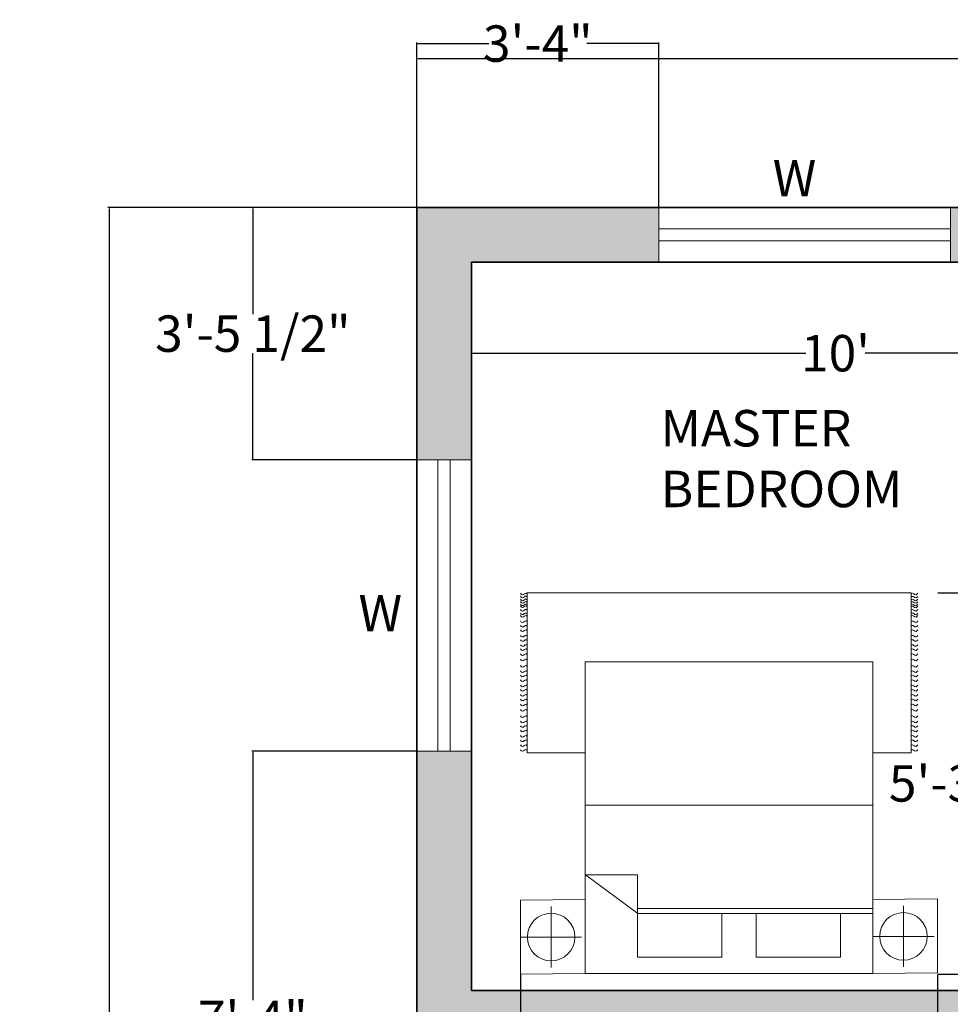
# Model space of a CAD drawing. Units: inches. Extents: x 302 to 1258, y 831 to 1373.
# Tile 9 of 13: x 781 to 934, y 1211 to 1373. Entities that reach past the tile are written whole.
import ezdxf

# ---------------------------------------------------------------- set-up
doc = ezdxf.new("R2010")
doc.units = ezdxf.units.IN
doc.header["$MEASUREMENT"] = 0
for name, color, linetype, lineweight in [('A-ANNO-DIMS', 2, 'Continuous', 18), ('A-ANNO-TEXT', 7, 'Continuous', 18), ('A-AREA-IDEN', 7, 'Continuous', 18), ('A-FURN', 8, 'Continuous', 18), ('A-GLAZ', 4, 'Continuous', 18), ('A-WALL', 7, 'Continuous', 35), ('A-WALL-PATT', 251, 'Continuous', 13)]:
    doc.layers.add(name, color=color, linetype=linetype, lineweight=lineweight)
doc.styles.get("Standard").update_dxf_attribs({"font": 'arial.ttf'})
doc.dimstyles.get("Standard").update_dxf_attribs({"dimtxt": 6, "dimasz": 0.18, "dimexe": 0.18, "dimexo": 0.0625, "dimgap": 0.09, "dimtad": 0, "dimtih": 1, "dimtoh": 1, "dimdec": 1, "dimzin": 0, "dimdsep": 46, "dimlunit": 3, "dimtxsty": 'Standard', "dimcen": 0.09, "dimadec": 0, "dimazin": 0, "dimtfac": 1, "dimtdec": 1, "dimtofl": 0, "dimtmove": 0, "dimatfit": 3, "dimfxl": 1, "dimtolj": 1, "dimtzin": 0, "dimarcsym": 0})

# ---------------------------------------------------------------- blocks, each defined once
blk = doc.blocks.new('*D17')
at = {"layer": 'A-ANNO-DIMS', "color": 0, "lineweight": -2, "transparency": 16777216}
for p, q in [((855.12, 1333.26), (855.12, 1318.14)), ((975.12, 1333.26), (975.12, 1318.14)), ((855.3, 1318.32), (910.22, 1318.32)), ((974.94, 1318.32), (920.02, 1318.32))]:
    blk.add_line(p, q, dxfattribs=at)
at = {"layer": 'A-ANNO-DIMS', "color": 0, "transparency": 16777216}
for points in [[(855.3, 1318.35), (855.3, 1318.29), (855.12, 1318.32)], [(974.94, 1318.35), (974.94, 1318.29), (975.12, 1318.32)]]:
    blk.add_solid(points, dxfattribs=at)
at = {"layer": 'Defpoints', "color": 0, "transparency": 16777216}
for p in [(855.12, 1333.32), (975.12, 1333.32), (975.12, 1318.32)]:
    blk.add_point(p, dxfattribs=at)
at = {"layer": 'A-ANNO-DIMS', "color": 0, "transparency": 16777216, "insert": (915.12, 1318.32), "char_height": 6, "attachment_point": 5}
blk.add_mtext("\\A1;10'", dxfattribs=at)
blk = doc.blocks.new('*D33')
at = {"layer": 'A-ANNO-DIMS', "color": 0, "lineweight": -2, "transparency": 16777216}
for p, q in [((846.12, 1342.38), (846.12, 1367.04)), ((846.3, 1366.86), (1010.68, 1366.86)), ((1202.94, 1366.86), (1038.56, 1366.86)), ((1203.12, 1342.38), (1203.12, 1367.04))]:
    blk.add_line(p, q, dxfattribs=at)
at = {"layer": 'A-ANNO-DIMS', "color": 0, "transparency": 16777216}
for points in [[(846.3, 1366.89), (846.3, 1366.83), (846.12, 1366.86)], [(1202.94, 1366.89), (1202.94, 1366.83), (1203.12, 1366.86)]]:
    blk.add_solid(points, dxfattribs=at)
at = {"layer": 'Defpoints', "color": 0, "transparency": 16777216}
for p in [(1203.12, 1366.86), (846.12, 1342.32), (1203.12, 1342.32)]:
    blk.add_point(p, dxfattribs=at)
at = {"layer": 'A-ANNO-DIMS', "color": 0, "transparency": 16777216, "insert": (1024.62, 1366.86), "char_height": 6, "attachment_point": 5}
blk.add_mtext('\\A1;29\'-9.0"', dxfattribs=at)
blk = doc.blocks.new('*D34')
at = {"layer": 'A-ANNO-DIMS', "color": 0, "lineweight": -2, "transparency": 16777216}
for p, q in [((846.06, 1342.32), (795.24, 1342.32)), ((795.42, 1342.14), (795.42, 1107.72)), ((795.42, 867), (795.42, 1101.41)), ((846.06, 866.82), (795.24, 866.82))]:
    blk.add_line(p, q, dxfattribs=at)
at = {"layer": 'A-ANNO-DIMS', "color": 0, "transparency": 16777216}
for points in [[(795.39, 1342.14), (795.45, 1342.14), (795.42, 1342.32)], [(795.39, 867), (795.45, 867), (795.42, 866.82)]]:
    blk.add_solid(points, dxfattribs=at)
at = {"layer": 'Defpoints', "color": 0, "transparency": 16777216}
for p in [(846.12, 1342.32), (795.42, 866.82), (846.12, 866.82)]:
    blk.add_point(p, dxfattribs=at)
at = {"layer": 'A-ANNO-DIMS', "color": 0, "transparency": 16777216, "insert": (795.42, 1104.57), "char_height": 6, "attachment_point": 5}
blk.add_mtext('\\A1;39\'-7.5"', dxfattribs=at)
blk = doc.blocks.new('BED-DOUBLE-WITH-NIGHTSTANDS')
for p, q in [((1.12, 36.41), (1.12, 62.78)), ((1.12, 62.78), (64.36, 62.78)), ((64.36, 62.78), (64.36, 36.41)), ((10.66, 36.41), (1.12, 36.41)), ((64.36, 36.41), (58.06, 36.41)), ((10.66, 27.82), (58.08, 27.82)), ((19.27, 16.32), (10.71, 16.32)), ((19.32, 9.97), (10.71, 16.32)), ((19.27, 9.97), (19.27, 16.32)), ((5.06, 1.07), (5.06, 11.12)), ((19.27, 10.78), (58.08, 10.78)), ((19.32, 9.97), (58.08, 9.97)), ((63.11, 1.17), (63.11, 11.22)), ((0.03, 6.09), (10.09, 6.09)), ((58.08, 6.2), (68.14, 6.2))]:
    blk.add_line(p, q)
for points in [[(10.66, 0.1), (10.66, 51.42), (58.08, 51.42), (58.08, 0.1)], [(10.66, 12.29), (0.03, 12.19), (0.03, 0), (10.66, 0.1)], [(68.71, 12.39), (58.08, 12.29), (58.08, 0.1), (68.71, 0.2)], [(19.27, 2.8), (19.27, 9.97), (33.16, 9.97), (33.16, 2.8)], [(38.83, 2.8), (38.83, 9.97), (52.73, 9.97), (52.73, 2.8)]]:
    blk.add_lwpolyline(points, close=True)
for centre in [(5.06, 6.09), (63.11, 6.2)]:
    blk.add_circle(centre, 3.92)
for points, knots in [([(0, 62.71), (0.1, 62.59), (0.29, 62.35), (0.63, 62.59), (0.91, 62.76), (1.06, 62.66), (1.13, 62.61)], [0, 0, 0, 0, 0.400747, 0.791423, 1.067667, 1.29709, 1.29709, 1.29709, 1.29709]), ([(0, 62.24), (0.1, 62.12), (0.29, 61.88), (0.63, 62.12), (0.91, 62.29), (1.06, 62.18), (1.13, 62.13)], [0, 0, 0, 0, 0.400747, 0.791423, 1.067667, 1.29709, 1.29709, 1.29709, 1.29709]), ([(0, 61.75), (0.1, 61.63), (0.29, 61.39), (0.63, 61.63), (0.91, 61.8), (1.06, 61.7), (1.13, 61.65)], [0, 0, 0, 0, 0.400747, 0.791423, 1.067667, 1.29709, 1.29709, 1.29709, 1.29709]), ([(65.48, 62.71), (65.39, 62.59), (65.19, 62.35), (64.85, 62.59), (64.57, 62.76), (64.42, 62.66), (64.36, 62.61)], [0, 0, 0, 0, 0.400747, 0.791423, 1.067667, 1.29709, 1.29709, 1.29709, 1.29709]), ([(65.48, 62.21), (65.39, 62.09), (65.19, 61.85), (64.85, 62.09), (64.57, 62.26), (64.42, 62.15), (64.36, 62.11)], [0, 0, 0, 0, 0.400747, 0.791423, 1.067667, 1.29709, 1.29709, 1.29709, 1.29709]), ([(65.48, 61.72), (65.39, 61.6), (65.19, 61.36), (64.85, 61.6), (64.57, 61.78), (64.42, 61.67), (64.36, 61.62)], [0, 0, 0, 0, 0.400747, 0.791423, 1.067667, 1.29709, 1.29709, 1.29709, 1.29709]), ([(0, 61.35), (0.1, 61.23), (0.29, 60.99), (0.63, 61.23), (0.91, 61.41), (1.06, 61.3), (1.13, 61.25)], [0, 0, 0, 0, 0.400747, 0.791423, 1.067667, 1.29709, 1.29709, 1.29709, 1.29709]), ([(0, 60.94), (0.1, 60.81), (0.29, 60.58), (0.63, 60.81), (0.91, 60.99), (1.05, 60.89), (1.12, 60.84)], [0, 0, 0, 0, 0.400747, 0.791423, 1.067667, 1.283686, 1.283686, 1.283686, 1.283686]), ([(0, 60.63), (0.1, 60.51), (0.29, 60.27), (0.63, 60.51), (0.91, 60.68), (1.05, 60.58), (1.12, 60.53)], [0, 0, 0, 0, 0.400747, 0.791423, 1.067667, 1.283686, 1.283686, 1.283686, 1.283686]), ([(0, 60.05), (0.1, 59.93), (0.29, 59.69), (0.63, 59.93), (0.91, 60.1), (1.05, 60), (1.12, 59.96)], [0, 0, 0, 0, 0.400747, 0.791423, 1.067667, 1.283686, 1.283686, 1.283686, 1.283686]), ([(65.48, 61.33), (65.39, 61.21), (65.19, 60.97), (64.85, 61.21), (64.57, 61.38), (64.42, 61.27), (64.36, 61.22)], [0, 0, 0, 0, 0.400747, 0.791423, 1.067667, 1.29709, 1.29709, 1.29709, 1.29709]), ([(65.48, 60.91), (65.39, 60.79), (65.19, 60.55), (64.85, 60.79), (64.57, 60.96), (64.42, 60.85), (64.36, 60.81)], [0, 0, 0, 0, 0.400747, 0.791423, 1.067667, 1.29709, 1.29709, 1.29709, 1.29709]), ([(65.48, 60.6), (65.39, 60.48), (65.19, 60.24), (64.85, 60.48), (64.57, 60.65), (64.42, 60.54), (64.36, 60.5)], [0, 0, 0, 0, 0.400747, 0.791423, 1.067667, 1.29709, 1.29709, 1.29709, 1.29709]), ([(65.48, 60.03), (65.39, 59.9), (65.19, 59.67), (64.85, 59.9), (64.57, 60.08), (64.42, 59.97), (64.36, 59.92)], [0, 0, 0, 0, 0.400747, 0.791423, 1.067667, 1.29709, 1.29709, 1.29709, 1.29709]), ([(0, 59.46), (0.1, 59.34), (0.29, 59.09), (0.63, 59.34), (0.91, 59.51), (1.05, 59.41), (1.12, 59.36)], [0, 0, 0, 0, 0.402903, 0.794912, 1.071156, 1.287177, 1.287177, 1.287177, 1.287177]), ([(0, 59.03), (0.1, 58.91), (0.29, 58.67), (0.63, 58.91), (0.91, 59.08), (1.05, 58.98), (1.12, 58.93)], [0, 0, 0, 0, 0.400747, 0.791423, 1.067667, 1.283686, 1.283686, 1.283686, 1.283686]), ([(65.48, 59.46), (65.39, 59.33), (65.2, 59.08), (64.85, 59.34), (64.57, 59.51), (64.42, 59.4), (64.36, 59.36)], [0, 0, 0, 0, 0.407265, 0.802015, 1.07826, 1.307683, 1.307683, 1.307683, 1.307683]), ([(65.48, 59.03), (65.39, 58.91), (65.19, 58.67), (64.85, 58.91), (64.57, 59.08), (64.42, 58.97), (64.36, 58.93)], [0, 0, 0, 0, 0.400747, 0.791423, 1.067667, 1.29709, 1.29709, 1.29709, 1.29709]), ([(0, 58.15), (0.1, 58.03), (0.29, 57.79), (0.63, 58.03), (0.91, 58.2), (1.05, 58.1), (1.12, 58.05)], [0, 0, 0, 0, 0.400747, 0.791423, 1.067667, 1.283686, 1.283686, 1.283686, 1.283686]), ([(0, 57.42), (0.1, 57.3), (0.29, 57.06), (0.63, 57.3), (0.91, 57.47), (1.06, 57.36), (1.13, 57.32)], [0, 0, 0, 0, 0.400747, 0.791423, 1.067667, 1.29709, 1.29709, 1.29709, 1.29709]), ([(65.48, 58.15), (65.39, 58.03), (65.19, 57.79), (64.85, 58.03), (64.57, 58.2), (64.42, 58.09), (64.36, 58.04)], [0, 0, 0, 0, 0.400747, 0.791423, 1.067667, 1.29709, 1.29709, 1.29709, 1.29709]), ([(65.48, 57.42), (65.39, 57.3), (65.19, 57.06), (64.85, 57.3), (64.57, 57.47), (64.42, 57.36), (64.36, 57.32)], [0, 0, 0, 0, 0.400747, 0.791423, 1.067667, 1.29709, 1.29709, 1.29709, 1.29709]), ([(0, 56.67), (0.1, 56.55), (0.29, 56.31), (0.63, 56.55), (0.91, 56.72), (1.06, 56.61), (1.13, 56.56)], [0, 0, 0, 0, 0.400747, 0.791423, 1.067667, 1.29709, 1.29709, 1.29709, 1.29709]), ([(0, 55.78), (0.1, 55.66), (0.29, 55.42), (0.63, 55.66), (0.91, 55.84), (1.06, 55.73), (1.13, 55.68)], [0, 0, 0, 0, 0.400747, 0.791423, 1.067667, 1.29709, 1.29709, 1.29709, 1.29709]), ([(65.48, 56.67), (65.39, 56.55), (65.19, 56.31), (64.85, 56.55), (64.57, 56.72), (64.42, 56.61), (64.36, 56.56)], [0, 0, 0, 0, 0.400747, 0.791423, 1.067667, 1.29709, 1.29709, 1.29709, 1.29709]), ([(65.48, 55.78), (65.39, 55.66), (65.19, 55.42), (64.85, 55.66), (64.57, 55.84), (64.42, 55.73), (64.36, 55.68)], [0, 0, 0, 0, 0.400747, 0.791423, 1.067667, 1.29709, 1.29709, 1.29709, 1.29709]), ([(0, 55.06), (0.1, 54.94), (0.29, 54.7), (0.63, 54.94), (0.91, 55.11), (1.06, 55), (1.13, 54.95)], [0, 0, 0, 0, 0.400747, 0.791423, 1.067667, 1.29709, 1.29709, 1.29709, 1.29709]), ([(0, 54.24), (0.1, 54.12), (0.29, 53.88), (0.63, 54.12), (0.91, 54.29), (1.06, 54.19), (1.13, 54.14)], [0, 0, 0, 0, 0.400747, 0.791423, 1.067667, 1.29709, 1.29709, 1.29709, 1.29709]), ([(0, 53.55), (0.1, 53.43), (0.29, 53.19), (0.63, 53.43), (0.91, 53.6), (1.06, 53.5), (1.13, 53.45)], [0, 0, 0, 0, 0.400747, 0.791423, 1.067667, 1.29709, 1.29709, 1.29709, 1.29709]), ([(65.48, 55.06), (65.39, 54.94), (65.19, 54.7), (64.85, 54.94), (64.57, 55.11), (64.42, 55), (64.36, 54.95)], [0, 0, 0, 0, 0.400747, 0.791423, 1.067667, 1.29709, 1.29709, 1.29709, 1.29709]), ([(65.48, 54.24), (65.39, 54.12), (65.19, 53.88), (64.85, 54.12), (64.57, 54.29), (64.42, 54.19), (64.36, 54.14)], [0, 0, 0, 0, 0.400747, 0.791423, 1.067667, 1.29709, 1.29709, 1.29709, 1.29709]), ([(65.48, 53.55), (65.39, 53.43), (65.19, 53.19), (64.85, 53.43), (64.57, 53.6), (64.42, 53.5), (64.36, 53.45)], [0, 0, 0, 0, 0.400747, 0.791423, 1.067667, 1.29709, 1.29709, 1.29709, 1.29709]), ([(0, 52.73), (0.1, 52.61), (0.29, 52.37), (0.63, 52.61), (0.91, 52.79), (1.06, 52.68), (1.13, 52.63)], [0, 0, 0, 0, 0.400747, 0.791423, 1.067667, 1.29709, 1.29709, 1.29709, 1.29709]), ([(65.48, 52.73), (65.39, 52.61), (65.19, 52.37), (64.85, 52.61), (64.57, 52.79), (64.42, 52.68), (64.36, 52.63)], [0, 0, 0, 0, 0.400747, 0.791423, 1.067667, 1.29709, 1.29709, 1.29709, 1.29709]), ([(0, 51.85), (0.1, 51.73), (0.29, 51.49), (0.63, 51.73), (0.91, 51.9), (1.06, 51.8), (1.13, 51.75)], [0, 0, 0, 0, 0.400747, 0.791423, 1.067667, 1.29709, 1.29709, 1.29709, 1.29709]), ([(0, 50.82), (0.1, 50.69), (0.29, 50.46), (0.63, 50.69), (0.91, 50.87), (1.06, 50.76), (1.13, 50.71)], [0, 0, 0, 0, 0.400747, 0.791423, 1.067667, 1.29709, 1.29709, 1.29709, 1.29709]), ([(65.48, 51.85), (65.39, 51.73), (65.19, 51.49), (64.85, 51.73), (64.57, 51.9), (64.42, 51.8), (64.36, 51.75)], [0, 0, 0, 0, 0.400747, 0.791423, 1.067667, 1.29709, 1.29709, 1.29709, 1.29709]), ([(65.48, 50.82), (65.39, 50.69), (65.19, 50.46), (64.85, 50.69), (64.57, 50.87), (64.42, 50.76), (64.36, 50.71)], [0, 0, 0, 0, 0.400747, 0.791423, 1.067667, 1.29709, 1.29709, 1.29709, 1.29709]), ([(0, 49.93), (0.1, 49.81), (0.29, 49.57), (0.63, 49.81), (0.91, 49.99), (1.06, 49.88), (1.13, 49.83)], [0, 0, 0, 0, 0.400747, 0.791423, 1.067667, 1.29709, 1.29709, 1.29709, 1.29709]), ([(0, 49.21), (0.1, 49.08), (0.29, 48.84), (0.63, 49.08), (0.91, 49.26), (1.06, 49.15), (1.13, 49.1)], [0, 0, 0, 0, 0.400747, 0.791423, 1.067667, 1.29709, 1.29709, 1.29709, 1.29709]), ([(65.48, 49.93), (65.39, 49.81), (65.19, 49.57), (64.85, 49.81), (64.57, 49.99), (64.42, 49.88), (64.36, 49.83)], [0, 0, 0, 0, 0.400747, 0.791423, 1.067667, 1.29709, 1.29709, 1.29709, 1.29709]), ([(65.48, 49.21), (65.39, 49.08), (65.19, 48.84), (64.85, 49.08), (64.57, 49.26), (64.42, 49.15), (64.36, 49.1)], [0, 0, 0, 0, 0.400747, 0.791423, 1.067667, 1.29709, 1.29709, 1.29709, 1.29709]), ([(0, 48.45), (0.1, 48.33), (0.29, 48.09), (0.63, 48.33), (0.91, 48.51), (1.06, 48.4), (1.13, 48.35)], [0, 0, 0, 0, 0.400747, 0.791423, 1.067667, 1.29709, 1.29709, 1.29709, 1.29709]), ([(0, 47.57), (0.1, 47.45), (0.29, 47.21), (0.63, 47.45), (0.91, 47.62), (1.06, 47.52), (1.13, 47.47)], [0, 0, 0, 0, 0.400747, 0.791423, 1.067667, 1.29709, 1.29709, 1.29709, 1.29709]), ([(65.48, 48.45), (65.39, 48.33), (65.19, 48.09), (64.85, 48.33), (64.57, 48.51), (64.42, 48.4), (64.36, 48.35)], [0, 0, 0, 0, 0.400747, 0.791423, 1.067667, 1.29709, 1.29709, 1.29709, 1.29709]), ([(65.48, 47.57), (65.39, 47.45), (65.19, 47.21), (64.85, 47.45), (64.57, 47.62), (64.42, 47.52), (64.36, 47.47)], [0, 0, 0, 0, 0.400747, 0.791423, 1.067667, 1.29709, 1.29709, 1.29709, 1.29709]), ([(0, 46.84), (0.1, 46.72), (0.29, 46.48), (0.63, 46.72), (0.91, 46.89), (1.06, 46.79), (1.13, 46.74)], [0, 0, 0, 0, 0.400747, 0.791423, 1.067667, 1.29709, 1.29709, 1.29709, 1.29709]), ([(0, 46.03), (0.1, 45.91), (0.29, 45.67), (0.63, 45.91), (0.91, 46.08), (1.06, 45.97), (1.13, 45.92)], [0, 0, 0, 0, 0.400747, 0.791423, 1.067667, 1.29709, 1.29709, 1.29709, 1.29709]), ([(65.48, 46.84), (65.39, 46.72), (65.19, 46.48), (64.85, 46.72), (64.57, 46.89), (64.42, 46.79), (64.36, 46.74)], [0, 0, 0, 0, 0.400747, 0.791423, 1.067667, 1.29709, 1.29709, 1.29709, 1.29709]), ([(65.48, 46.03), (65.39, 45.91), (65.19, 45.67), (64.85, 45.91), (64.57, 46.08), (64.42, 45.97), (64.36, 45.92)], [0, 0, 0, 0, 0.400747, 0.791423, 1.067667, 1.29709, 1.29709, 1.29709, 1.29709]), ([(0, 45.25), (0.1, 45.13), (0.29, 44.89), (0.63, 45.13), (0.91, 45.3), (1.06, 45.2), (1.13, 45.15)], [0, 0, 0, 0, 0.400747, 0.791423, 1.067667, 1.29709, 1.29709, 1.29709, 1.29709]), ([(0, 44.43), (0.1, 44.31), (0.29, 44.07), (0.63, 44.31), (0.91, 44.49), (1.06, 44.38), (1.13, 44.33)], [0, 0, 0, 0, 0.400747, 0.791423, 1.067667, 1.29709, 1.29709, 1.29709, 1.29709]), ([(65.48, 45.25), (65.39, 45.13), (65.19, 44.89), (64.85, 45.13), (64.57, 45.3), (64.42, 45.2), (64.36, 45.15)], [0, 0, 0, 0, 0.400747, 0.791423, 1.067667, 1.29709, 1.29709, 1.29709, 1.29709]), ([(65.48, 44.43), (65.39, 44.31), (65.19, 44.07), (64.85, 44.31), (64.57, 44.49), (64.42, 44.38), (64.36, 44.33)], [0, 0, 0, 0, 0.400747, 0.791423, 1.067667, 1.29709, 1.29709, 1.29709, 1.29709]), ([(0, 43.55), (0.1, 43.43), (0.29, 43.19), (0.63, 43.43), (0.91, 43.6), (1.06, 43.5), (1.13, 43.45)], [0, 0, 0, 0, 0.400747, 0.791423, 1.067667, 1.29709, 1.29709, 1.29709, 1.29709]), ([(0, 42.52), (0.1, 42.39), (0.29, 42.15), (0.63, 42.39), (0.91, 42.57), (1.06, 42.46), (1.13, 42.41)], [0, 0, 0, 0, 0.400747, 0.791423, 1.067667, 1.29709, 1.29709, 1.29709, 1.29709]), ([(65.48, 43.55), (65.39, 43.43), (65.19, 43.19), (64.85, 43.43), (64.57, 43.6), (64.42, 43.5), (64.36, 43.45)], [0, 0, 0, 0, 0.400747, 0.791423, 1.067667, 1.29709, 1.29709, 1.29709, 1.29709]), ([(65.48, 42.52), (65.39, 42.39), (65.19, 42.15), (64.85, 42.39), (64.57, 42.57), (64.42, 42.46), (64.36, 42.41)], [0, 0, 0, 0, 0.400747, 0.791423, 1.067667, 1.29709, 1.29709, 1.29709, 1.29709]), ([(0, 41.63), (0.1, 41.51), (0.29, 41.27), (0.63, 41.51), (0.91, 41.68), (1.06, 41.58), (1.13, 41.53)], [0, 0, 0, 0, 0.400747, 0.791423, 1.067667, 1.29709, 1.29709, 1.29709, 1.29709]), ([(0, 40.9), (0.1, 40.78), (0.29, 40.54), (0.63, 40.78), (0.91, 40.96), (1.06, 40.85), (1.13, 40.8)], [0, 0, 0, 0, 0.400747, 0.791423, 1.067667, 1.29709, 1.29709, 1.29709, 1.29709]), ([(65.48, 41.63), (65.39, 41.51), (65.19, 41.27), (64.85, 41.51), (64.57, 41.68), (64.42, 41.58), (64.36, 41.53)], [0, 0, 0, 0, 0.400747, 0.791423, 1.067667, 1.29709, 1.29709, 1.29709, 1.29709]), ([(65.48, 40.9), (65.39, 40.78), (65.19, 40.54), (64.85, 40.78), (64.57, 40.96), (64.42, 40.85), (64.36, 40.8)], [0, 0, 0, 0, 0.400747, 0.791423, 1.067667, 1.29709, 1.29709, 1.29709, 1.29709]), ([(0, 40.15), (0.1, 40.03), (0.29, 39.79), (0.63, 40.03), (0.91, 40.2), (1.06, 40.1), (1.13, 40.05)], [0, 0, 0, 0, 0.400747, 0.791423, 1.067667, 1.29709, 1.29709, 1.29709, 1.29709]), ([(0, 39.27), (0.1, 39.15), (0.29, 38.91), (0.63, 39.15), (0.91, 39.32), (1.06, 39.22), (1.13, 39.17)], [0, 0, 0, 0, 0.400747, 0.791423, 1.067667, 1.29709, 1.29709, 1.29709, 1.29709]), ([(65.48, 40.15), (65.39, 40.03), (65.19, 39.79), (64.85, 40.03), (64.57, 40.2), (64.42, 40.1), (64.36, 40.05)], [0, 0, 0, 0, 0.400747, 0.791423, 1.067667, 1.29709, 1.29709, 1.29709, 1.29709]), ([(65.48, 39.27), (65.39, 39.15), (65.19, 38.91), (64.85, 39.15), (64.57, 39.32), (64.42, 39.22), (64.36, 39.17)], [0, 0, 0, 0, 0.400747, 0.791423, 1.067667, 1.29709, 1.29709, 1.29709, 1.29709]), ([(0, 38.54), (0.1, 38.42), (0.29, 38.18), (0.63, 38.42), (0.91, 38.59), (1.06, 38.49), (1.13, 38.44)], [0, 0, 0, 0, 0.400747, 0.791423, 1.067667, 1.29709, 1.29709, 1.29709, 1.29709]), ([(0, 37.73), (0.1, 37.61), (0.29, 37.37), (0.63, 37.61), (0.91, 37.78), (1.06, 37.67), (1.13, 37.62)], [0, 0, 0, 0, 0.400747, 0.791423, 1.067667, 1.29709, 1.29709, 1.29709, 1.29709]), ([(65.48, 38.54), (65.39, 38.42), (65.19, 38.18), (64.85, 38.42), (64.57, 38.59), (64.42, 38.49), (64.36, 38.44)], [0, 0, 0, 0, 0.400747, 0.791423, 1.067667, 1.29709, 1.29709, 1.29709, 1.29709]), ([(65.48, 37.73), (65.39, 37.61), (65.19, 37.37), (64.85, 37.61), (64.57, 37.78), (64.42, 37.67), (64.36, 37.62)], [0, 0, 0, 0, 0.400747, 0.791423, 1.067667, 1.29709, 1.29709, 1.29709, 1.29709]), ([(0, 36.95), (0.1, 36.83), (0.29, 36.59), (0.63, 36.83), (0.91, 37), (1.06, 36.89), (1.13, 36.85)], [0, 0, 0, 0, 0.400747, 0.791423, 1.067667, 1.29709, 1.29709, 1.29709, 1.29709]), ([(65.48, 36.95), (65.39, 36.83), (65.19, 36.59), (64.85, 36.83), (64.57, 37), (64.42, 36.89), (64.36, 36.85)], [0, 0, 0, 0, 0.400747, 0.791423, 1.067667, 1.29709, 1.29709, 1.29709, 1.29709])]:
    blk.add_open_spline(points, degree=3, knots=knots)
blk = doc.blocks.new('WINDOW-48IN')
for p, q in [((0, 0), (0, 9)), ((0, 9), (48, 9)), ((48, 9), (48, 0)), ((0, 5.5), (48, 5.5)), ((48, 3.5), (0, 3.5)), ((48, 0), (0, 0))]:
    blk.add_line(p, q)
blk = doc.blocks.new('*D51')
at = {"layer": 'A-ANNO-DIMS', "color": 0, "lineweight": -2, "transparency": 16777216}
for p, q in [((863.2, 1216), (863.2, 1205.58)), ((931.91, 1216), (931.91, 1205.58)), ((863.38, 1205.76), (931.73, 1205.76)), ((931.91, 1205.76), (932.09, 1205.76))]:
    blk.add_line(p, q, dxfattribs=at)
at = {"layer": 'A-ANNO-DIMS', "color": 0, "transparency": 16777216}
for points in [[(863.38, 1205.79), (863.38, 1205.73), (863.2, 1205.76)], [(931.73, 1205.79), (931.73, 1205.73), (931.91, 1205.76)]]:
    blk.add_solid(points, dxfattribs=at)
at = {"layer": 'Defpoints', "color": 0, "transparency": 16777216}
for p in [(863.2, 1216.06), (931.91, 1216.06), (931.91, 1205.76)]:
    blk.add_point(p, dxfattribs=at)
at = {"layer": 'A-ANNO-DIMS', "color": 0, "transparency": 16777216, "insert": (976.42, 1205.76), "char_height": 6, "attachment_point": 5}
blk.add_mtext('\\A1;BED SET 5\'-8 1/2" TYP.', dxfattribs=at)
blk = doc.blocks.new('*D52')
at = {"layer": 'A-ANNO-DIMS', "color": 0, "lineweight": -2, "transparency": 16777216}
for p, q in [((931.98, 1278.85), (942.4, 1278.85)), ((942.22, 1278.67), (942.22, 1250.61)), ((942.22, 1216.24), (942.22, 1244.3)), ((931.98, 1216.06), (942.4, 1216.06))]:
    blk.add_line(p, q, dxfattribs=at)
at = {"layer": 'A-ANNO-DIMS', "color": 0, "transparency": 16777216}
for points in [[(942.19, 1278.67), (942.25, 1278.67), (942.22, 1278.85)], [(942.19, 1216.24), (942.25, 1216.24), (942.22, 1216.06)]]:
    blk.add_solid(points, dxfattribs=at)
at = {"layer": 'Defpoints', "color": 0, "transparency": 16777216}
for p in [(931.91, 1278.85), (942.22, 1278.85), (931.91, 1216.06)]:
    blk.add_point(p, dxfattribs=at)
at = {"layer": 'A-ANNO-DIMS', "color": 0, "transparency": 16777216, "insert": (942.22, 1247.46), "char_height": 6, "attachment_point": 5}
blk.add_mtext('\\A1;5\'-3" TYP.', dxfattribs=at)
blk = doc.blocks.new('*D85')
at = {"layer": 'A-ANNO-DIMS', "color": 0, "lineweight": -2, "transparency": 16777216}
for p, q in [((846.12, 1342.38), (846.12, 1369.5)), ((846.3, 1369.32), (858.01, 1369.32)), ((885.85, 1369.32), (874.14, 1369.32)), ((886.03, 1342.38), (886.03, 1369.5))]:
    blk.add_line(p, q, dxfattribs=at)
at = {"layer": 'A-ANNO-DIMS', "color": 0, "transparency": 16777216}
for points in [[(846.3, 1369.35), (846.3, 1369.29), (846.12, 1369.32)], [(885.85, 1369.35), (885.85, 1369.29), (886.03, 1369.32)]]:
    blk.add_solid(points, dxfattribs=at)
at = {"layer": 'Defpoints', "color": 0, "transparency": 16777216}
for p in [(886.03, 1369.32), (846.12, 1342.32), (886.03, 1342.32)]:
    blk.add_point(p, dxfattribs=at)
at = {"layer": 'A-ANNO-DIMS', "color": 0, "transparency": 16777216, "insert": (866.07, 1369.32), "char_height": 6, "attachment_point": 5}
blk.add_mtext('\\A1;3\'-4"', dxfattribs=at)
blk = doc.blocks.new('*D87')
at = {"layer": 'A-ANNO-DIMS', "color": 0, "lineweight": -2, "transparency": 16777216}
for p, q in [((846.06, 1342.32), (818.94, 1342.32)), ((819.12, 1342.14), (819.12, 1324.73)), ((819.12, 1300.94), (819.12, 1318.34)), ((846.06, 1300.76), (818.94, 1300.76))]:
    blk.add_line(p, q, dxfattribs=at)
at = {"layer": 'A-ANNO-DIMS', "color": 0, "transparency": 16777216}
for points in [[(819.09, 1342.14), (819.15, 1342.14), (819.12, 1342.32)], [(819.09, 1300.94), (819.15, 1300.94), (819.12, 1300.76)]]:
    blk.add_solid(points, dxfattribs=at)
at = {"layer": 'Defpoints', "color": 0, "transparency": 16777216}
for p in [(846.12, 1342.32), (819.12, 1300.76), (846.12, 1300.76)]:
    blk.add_point(p, dxfattribs=at)
at = {"layer": 'A-ANNO-DIMS', "color": 0, "transparency": 16777216, "insert": (819.12, 1321.54), "char_height": 6, "attachment_point": 5}
blk.add_mtext('\\A1;3\'-5 1/2"', dxfattribs=at)
blk = doc.blocks.new('*D88')
at = {"layer": 'A-ANNO-DIMS', "color": 0, "lineweight": -2, "transparency": 16777216}
for p, q in [((846.05954, 1252.758966), (818.94204, 1252.758966)), ((819.12204, 1252.578966), (819.12204, 1211.744211)), ((819.12204, 1164.729456), (819.12204, 1205.564211)), ((846.05954, 1164.549456), (818.94204, 1164.549456))]:
    blk.add_line(p, q, dxfattribs=at)
at = {"layer": 'A-ANNO-DIMS', "color": 0, "transparency": 16777216}
for points in [[(819.09204, 1252.578966), (819.15204, 1252.578966), (819.12204, 1252.758966)], [(819.09204, 1164.729456), (819.15204, 1164.729456), (819.12204, 1164.549456)]]:
    blk.add_solid(points, dxfattribs=at)
at = {"layer": 'Defpoints', "color": 0, "transparency": 16777216}
for p in [(846.12204, 1252.758966), (819.12204, 1164.549456), (846.12204, 1164.549456)]:
    blk.add_point(p, dxfattribs=at)
at = {"layer": 'A-ANNO-DIMS', "color": 0, "transparency": 16777216, "insert": (819.12204, 1208.654211), "char_height": 6, "attachment_point": 5}
blk.add_mtext('\\A1;7\'-4"', dxfattribs=at)

msp = doc.modelspace()

# ---------------------------------------------------------------- hatches: boundary and pattern name
at = {"layer": 'A-WALL-PATT'}
h = msp.add_hatch(color=256, dxfattribs=at)
h.dxf.hatch_style = 1
h.paths.add_polyline_path([(1003.23, 1342.32), (934.03, 1342.32), (934.03, 1333.32), (975.12, 1333.32), (975.12, 1330.32), (979.62, 1330.32), (979.62, 1333.32), (1003.23, 1333.32)])
h.paths.add_polyline_path([(1203.12, 1342.32), (1027.23, 1342.32), (1027.23, 1333.32), (1045.62, 1333.32), (1045.62, 1213.32), (979.62, 1213.32), (979.62, 1306.32), (975.12, 1306.32), (975.12, 1213.32), (974.12, 1213.32), (974.12, 1208.82), (975.12, 1208.82), (1051.12, 1208.82), (1051.12, 1213.32), (1050.12, 1213.32), (1050.12, 1333.32), (1194.12, 1333.32), (1194.12, 1302.71), (1203.12, 1302.71)])
h.paths.add_polyline_path([(855.12, 1333.32), (886.03, 1333.32), (886.03, 1342.32), (846.12, 1342.32), (846.12, 1300.76), (855.12, 1300.76)])
h.paths.add_polyline_path([(938.12, 1213.32), (855.12, 1213.32), (855.12, 1252.76), (846.12, 1252.76), (846.12, 1164.55), (855.12, 1164.55), (855.12, 1208.82), (933.12, 1208.82), (933.12, 1082.82), (937.62, 1082.82), (937.62, 1208.82), (938.12, 1208.82)])
h.paths.add_polyline_path([(855.12, 1116.55), (846.12, 1116.55), (846.12, 1024.44), (855.12, 1024.44)])
h.paths.add_polyline_path([(855.12, 976.44), (846.12, 976.44), (846.12, 944.2), (855.12, 944.2)])

# ---------------------------------------------------------------- linework, layer by layer
at = {"layer": 'A-WALL'}
for p, q in [((846.12, 1342.32), (1203.12, 1342.32)), ((846.12, 1342.32), (846.12, 866.82)), ((855.12, 1333.32), (975.12, 1333.32)), ((855.12, 1333.32), (855.12, 1213.32)), ((855.12, 1213.32), (938.12, 1213.32))]:
    msp.add_line(p, q, dxfattribs=at)

# ---------------------------------------------------------------- block references
at = {"layer": 'A-FURN'}
msp.add_blockref('BED-DOUBLE-WITH-NIGHTSTANDS', (863.2, 1216.06), dxfattribs=at)
at = {"layer": 'A-GLAZ'}
for p, rotation in [((934.03, 1342.32), 180), ((846.12, 1300.76), 269.9999999999993)]:
    msp.add_blockref('WINDOW-48IN', p, dxfattribs=dict(at, rotation=rotation))

# ---------------------------------------------------------------- texts
at = {"layer": 'A-ANNO-TEXT', "char_height": 6, "attachment_point": 1}
for insert in [(904.76, 1350.15), (836.52, 1278.48)]:
    msp.add_mtext_dynamic_manual_height_columns('W', width=16.4894, gutter_width=30, heights=[0], dxfattribs=dict(at, insert=insert))
at = {"layer": 'A-AREA-IDEN', "insert": (886.3, 1308.96), "char_height": 6, "attachment_point": 1}
msp.add_mtext_dynamic_manual_height_columns('MASTER\\PBEDROOM', width=60.4741, gutter_width=30, heights=[0], dxfattribs=at)

# ---------------------------------------------------------------- dimensions: what is measured, and where the dimension line sits
at = {"layer": 'A-ANNO-DIMS'}
for base, p1, p2, override, picture, middle in [((886.03, 1369.32), (846.12, 1342.32), (886.03, 1342.32), {"dimdec": 1, "dimlfac": 1, "dimrnd": 0, "dimzin": 1, "dimdsep": 46, "dimlunit": 4, "dimfrac": 2}, '*D85', (866.07, 1369.32)), ((1203.12, 1366.86), (846.12, 1342.32), (1203.12, 1342.32), {"dimclrd": 0, "dimclre": 0, "dimclrt": 0}, '*D33', (1024.62, 1366.86)), ((975.12, 1318.32), (855.12, 1333.32), (975.12, 1333.32), {"dimclrd": 0, "dimclre": 0, "dimclrt": 0}, '*D17', (915.12, 1318.32))]:
    dim = msp.add_linear_dim(base=base, p1=p1, p2=p2, dimstyle='Standard', override=override, dxfattribs=at)
    dim.commit()
    dim.dimension.update_dxf_attribs({"geometry": picture, "text_midpoint": middle})
for base, p1, p2, override, picture, middle in [((795.42, 866.82), (846.12, 1342.32), (846.12, 866.82), {"dimclrd": 0, "dimclre": 0, "dimclrt": 0}, '*D34', (795.42, 1104.57)), ((819.12, 1300.76), (846.12, 1342.32), (846.12, 1300.76), {"dimdec": 1, "dimlfac": 1, "dimrnd": 0, "dimzin": 1, "dimdsep": 46, "dimlunit": 4, "dimfrac": 2}, '*D87', (819.12, 1321.54)), ((819.12, 1164.55), (846.12, 1252.76), (846.12, 1164.55), {"dimdec": 1, "dimlfac": 1, "dimrnd": 0, "dimzin": 1, "dimdsep": 46, "dimlunit": 4, "dimfrac": 2}, '*D88', (819.12, 1208.65))]:
    dim = msp.add_linear_dim(base=base, p1=p1, p2=p2, angle=90, dimstyle='Standard', override=override, dxfattribs=at)
    dim.commit()
    dim.dimension.update_dxf_attribs({"geometry": picture, "text_midpoint": middle})
dim = msp.add_linear_dim(base=(942.22, 1278.85), p1=(931.91, 1216.06), p2=(931.91, 1278.85), angle=90, text='<> TYP.', dimstyle='Standard', override={"dimdec": 1, "dimlfac": 1, "dimrnd": 0, "dimzin": 1, "dimdsep": 46, "dimlunit": 4, "dimfrac": 2}, dxfattribs=at)
dim.commit()
dim.dimension.update_dxf_attribs({"geometry": '*D52', "text_midpoint": (942.22, 1247.46)})
dim = msp.add_linear_dim(base=(931.91, 1205.76), p1=(863.2, 1216.06), p2=(931.91, 1216.06), text='BED SET <> TYP.', dimstyle='Standard', override={"dimdec": 1, "dimlfac": 1, "dimrnd": 0, "dimzin": 1, "dimdsep": 46, "dimlunit": 4, "dimfrac": 2}, dxfattribs=at)
dim.commit()
dim.dimension.update_dxf_attribs({"geometry": '*D51', "text_midpoint": (976.42, 1205.76)})

doc.saveas('drawing.dxf')
